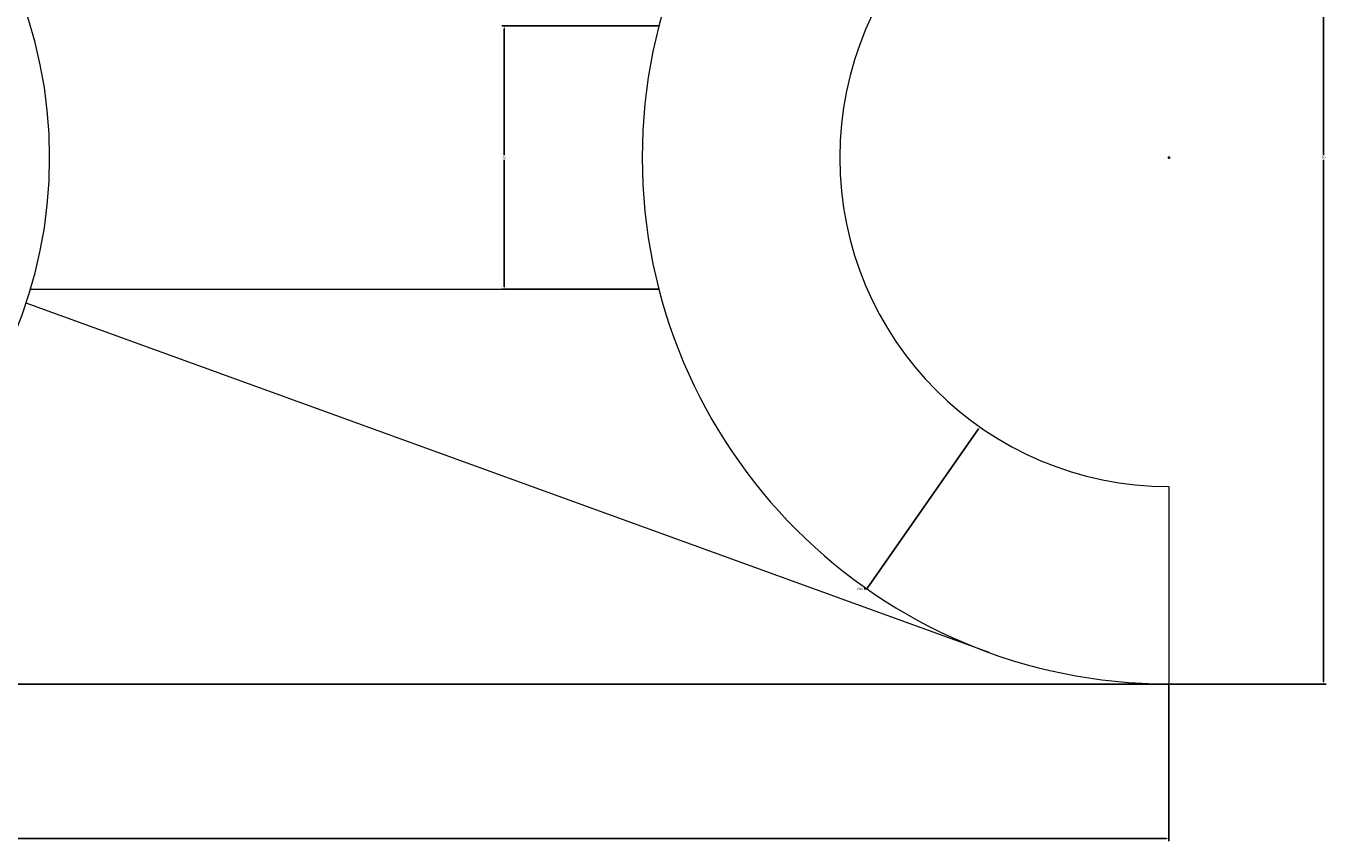
# Model space of a CAD drawing. Units: millimetres. Extents: x 3108 to 3332, y 1482 to 1586.
# Tile 4 of 5: x 3233 to 3332, y 1482 to 1544. Entities that reach past the tile are written whole.
import ezdxf

# ---------------------------------------------------------------- set-up
doc = ezdxf.new("R2010")
doc.units = ezdxf.units.MM
doc.layers.add('M-CONS', color=8, linetype='Continuous', lineweight=18)
doc.layers.add('M-DIMS', color=2, linetype='Continuous', lineweight=18)
doc.styles.get("Standard").update_dxf_attribs({"font": 'arial.ttf'})
doc.dimstyles.get("Standard").update_dxf_attribs({"dimtxt": 0.18, "dimasz": 0.18, "dimexe": 0.18, "dimexo": 0.0625, "dimgap": 0.09, "dimtad": 0, "dimtih": 1, "dimtoh": 1, "dimdec": 4, "dimzin": 0, "dimdsep": 46, "dimtxsty": 'Standard', "dimcen": 0.09, "dimadec": 0, "dimazin": 0, "dimtfac": 1, "dimtdec": 4, "dimtofl": 0, "dimtmove": 0, "dimatfit": 3, "dimfxl": 1, "dimtolj": 1, "dimtzin": 0, "dimarcsym": 0})

# ---------------------------------------------------------------- blocks, each defined once
blk = doc.blocks.new('*D1')
at = {"layer": 'Defpoints', "color": 0, "transparency": 16777216}
for p in [(3119.945, 1498.943), (3319.945, 1493.943), (3319.945, 1482.193)]:
    blk.add_point(p, dxfattribs=at)
at = {"layer": 'M-DIMS', "color": 0, "lineweight": -2, "transparency": 16777216}
for p, q in [((3119.945, 1498.881), (3119.945, 1482.013)), ((3319.945, 1493.881), (3319.945, 1482.013)), ((3120.125, 1482.193), (3219.655, 1482.193)), ((3319.765, 1482.193), (3220.235, 1482.193))]:
    blk.add_line(p, q, dxfattribs=at)
at = {"layer": 'M-DIMS', "color": 0, "transparency": 16777216}
for points in [[(3120.125, 1482.223), (3120.125, 1482.163), (3119.945, 1482.193)], [(3319.765, 1482.223), (3319.765, 1482.163), (3319.945, 1482.193)]]:
    blk.add_solid(points, dxfattribs=at)
at = {"layer": 'M-DIMS', "color": 0, "transparency": 16777216, "insert": (3219.945, 1482.193), "char_height": 0.18, "attachment_point": 5}
blk.add_mtext('\\A1;200', dxfattribs=at)
blk = doc.blocks.new('*D2')
at = {"layer": 'Defpoints', "color": 0, "transparency": 16777216}
for p in [(3319.945, 1573.943), (3331.695, 1573.943), (3319.945, 1493.943)]:
    blk.add_point(p, dxfattribs=at)
at = {"layer": 'M-DIMS', "color": 0, "lineweight": -2, "transparency": 16777216}
for p, q in [((3320.007, 1573.943), (3331.875, 1573.943)), ((3331.695, 1573.763), (3331.695, 1534.125)), ((3331.695, 1494.123), (3331.695, 1533.761)), ((3320.007, 1493.943), (3331.875, 1493.943))]:
    blk.add_line(p, q, dxfattribs=at)
at = {"layer": 'M-DIMS', "color": 0, "transparency": 16777216}
for points in [[(3331.665, 1573.763), (3331.725, 1573.763), (3331.695, 1573.943)], [(3331.665, 1494.123), (3331.725, 1494.123), (3331.695, 1493.943)]]:
    blk.add_solid(points, dxfattribs=at)
at = {"layer": 'M-DIMS', "color": 0, "transparency": 16777216, "insert": (3331.695, 1533.943), "char_height": 0.18, "attachment_point": 5}
blk.add_mtext('\\A1;80', dxfattribs=at)
blk = doc.blocks.new('*D7')
at = {"layer": 'Defpoints', "color": 0, "transparency": 16777216}
for p in [(3269.465, 1543.943), (3281.215, 1543.943), (3281.215, 1523.943)]:
    blk.add_point(p, dxfattribs=at)
at = {"layer": 'M-DIMS', "color": 0, "lineweight": -2, "transparency": 16777216}
for p, q in [((3281.152, 1543.943), (3269.285, 1543.943)), ((3269.465, 1543.763), (3269.465, 1534.125)), ((3269.465, 1524.123), (3269.465, 1533.761)), ((3281.152, 1523.943), (3269.285, 1523.943))]:
    blk.add_line(p, q, dxfattribs=at)
at = {"layer": 'M-DIMS', "color": 0, "transparency": 16777216}
for points in [[(3269.435, 1543.763), (3269.495, 1543.763), (3269.465, 1543.943)], [(3269.435, 1524.123), (3269.495, 1524.123), (3269.465, 1523.943)]]:
    blk.add_solid(points, dxfattribs=at)
at = {"layer": 'M-DIMS', "color": 0, "transparency": 16777216, "insert": (3269.465, 1533.943), "char_height": 0.18, "attachment_point": 5}
blk.add_mtext('\\A1;20', dxfattribs=at)
blk = doc.blocks.new('*D10')
at = {"layer": 'Defpoints', "color": 0, "transparency": 16777216}
for p in [(3119.945, 1498.943), (3108.195, 1493.943), (3319.945, 1493.943)]:
    blk.add_point(p, dxfattribs=at)
at = {"layer": 'M-DIMS', "color": 0, "lineweight": -2, "transparency": 16777216}
for p, q in [((3119.882, 1498.943), (3108.015, 1498.943)), ((3108.195, 1498.763), (3108.195, 1496.625)), ((3108.195, 1494.123), (3108.195, 1496.262)), ((3319.882, 1493.943), (3108.015, 1493.943))]:
    blk.add_line(p, q, dxfattribs=at)
at = {"layer": 'M-DIMS', "color": 0, "transparency": 16777216}
for points in [[(3108.165, 1498.763), (3108.225, 1498.763), (3108.195, 1498.943)], [(3108.165, 1494.123), (3108.225, 1494.123), (3108.195, 1493.943)]]:
    blk.add_solid(points, dxfattribs=at)
at = {"layer": 'M-DIMS', "color": 0, "transparency": 16777216, "insert": (3108.195, 1496.443), "char_height": 0.18, "attachment_point": 5}
blk.add_mtext('\\A1;5', dxfattribs=at)
blk = doc.blocks.new('*D11')
at = {"layer": 'Defpoints', "color": 0, "transparency": 16777216}
for p in [(3290.018, 1560.484), (3319.945, 1533.943)]:
    blk.add_point(p, dxfattribs=at)
at = {"layer": 'M-DIMS', "color": 0, "lineweight": -2, "transparency": 16777216}
for p, q in [((3271.882, 1576.408), (3272.062, 1576.408)), ((3272.062, 1576.408), (3289.884, 1560.603)), ((3319.855, 1533.943), (3320.035, 1533.943)), ((3319.945, 1533.853), (3319.945, 1534.033))]:
    blk.add_line(p, q, dxfattribs=at)
at = {"layer": 'M-DIMS', "color": 0, "transparency": 16777216}
blk.add_solid([(3289.904, 1560.626), (3289.864, 1560.581), (3290.018, 1560.484)], dxfattribs=at)
at = {"layer": 'M-DIMS', "color": 0, "transparency": 16777216, "insert": (3271.578, 1576.408), "char_height": 0.18, "attachment_point": 5}
blk.add_mtext('\\A1;R40', dxfattribs=at)
blk = doc.blocks.new('*D13')
at = {"layer": 'Defpoints', "color": 0, "transparency": 16777216}
for p in [(3319.945, 1533.943), (3305.599, 1513.469)]:
    blk.add_point(p, dxfattribs=at)
at = {"layer": 'M-DIMS', "color": 0, "lineweight": -2, "transparency": 16777216}
for p, q in [((3319.855, 1533.943), (3320.035, 1533.943)), ((3319.945, 1533.853), (3319.945, 1534.033)), ((3296.992, 1501.184), (3305.496, 1513.321)), ((3296.812, 1501.184), (3296.992, 1501.184))]:
    blk.add_line(p, q, dxfattribs=at)
at = {"layer": 'M-DIMS', "color": 0, "transparency": 16777216}
blk.add_solid([(3305.471, 1513.338), (3305.52, 1513.304), (3305.599, 1513.469)], dxfattribs=at)
at = {"layer": 'M-DIMS', "color": 0, "transparency": 16777216, "insert": (3296.506, 1501.184), "char_height": 0.18, "attachment_point": 5}
blk.add_mtext('\\A1;R25', dxfattribs=at)

msp = doc.modelspace()

# ---------------------------------------------------------------- linework, layer by layer
at = {"layer": 'M-CONS'}
for p, q in [((3233.4858, 1523.9431), (3281.2149, 1523.9431)), ((3306.3058, 1496.3402), (3233.1487, 1522.8751)), ((3319.9448, 1508.9431), (3319.9448, 1493.9431))]:
    msp.add_line(p, q, dxfattribs=at)
for centre, radius, start, end in [((3319.9448, 1533.9431), 40, 90, 270), ((3199.9448, 1533.9431), 35, 270, 90), ((3319.9448, 1533.9431), 25, 90, 270)]:
    msp.add_arc(centre, radius, start, end, dxfattribs=at)

# ---------------------------------------------------------------- dimensions: what is measured, and where the dimension line sits
at = {"layer": 'M-DIMS'}
for mpoint, picture, middle in [((3290.0183, 1560.4838), '*D11', (3271.5777, 1576.4082)), ((3305.5991, 1513.4687), '*D13', (3296.5059, 1501.184))]:
    dim = msp.add_radius_dim(center=(3319.9448, 1533.9431), mpoint=mpoint, dimstyle='Standard', override={"dimdec": 0, "dimlfac": 1, "dimrnd": 0, "dimzin": 0, "dimdsep": 46, "dimlunit": 2}, dxfattribs=at)
    dim.commit()
    dim.dimension.update_dxf_attribs({"geometry": picture, "text_midpoint": middle, "dimtype": 164})
for base, p1, p2, picture, middle in [((3331.6948, 1573.9431), (3319.9448, 1493.9431), (3319.9448, 1573.9431), '*D2', (3331.6948, 1533.9431)), ((3269.4649, 1543.9431), (3281.2149, 1523.9431), (3281.2149, 1543.9431), '*D7', (3269.4649, 1533.9431)), ((3108.1948, 1493.9431), (3119.9448, 1498.9431), (3319.9448, 1493.9431), '*D10', (3108.1948, 1496.4431))]:
    dim = msp.add_linear_dim(base=base, p1=p1, p2=p2, angle=90, dimstyle='Standard', override={"dimdec": 0, "dimlfac": 1, "dimrnd": 0, "dimzin": 0, "dimdsep": 46, "dimlunit": 2}, dxfattribs=at)
    dim.commit()
    dim.dimension.update_dxf_attribs({"geometry": picture, "text_midpoint": middle})
dim = msp.add_linear_dim(base=(3319.9448, 1482.1931), p1=(3119.9448, 1498.9431), p2=(3319.9448, 1493.9431), dimstyle='Standard', override={"dimdec": 0, "dimlfac": 1, "dimrnd": 0, "dimzin": 0, "dimdsep": 46, "dimlunit": 2}, dxfattribs=at)
dim.commit()
dim.dimension.update_dxf_attribs({"geometry": '*D1', "text_midpoint": (3219.9448, 1482.1931)})

doc.saveas('drawing.dxf')
